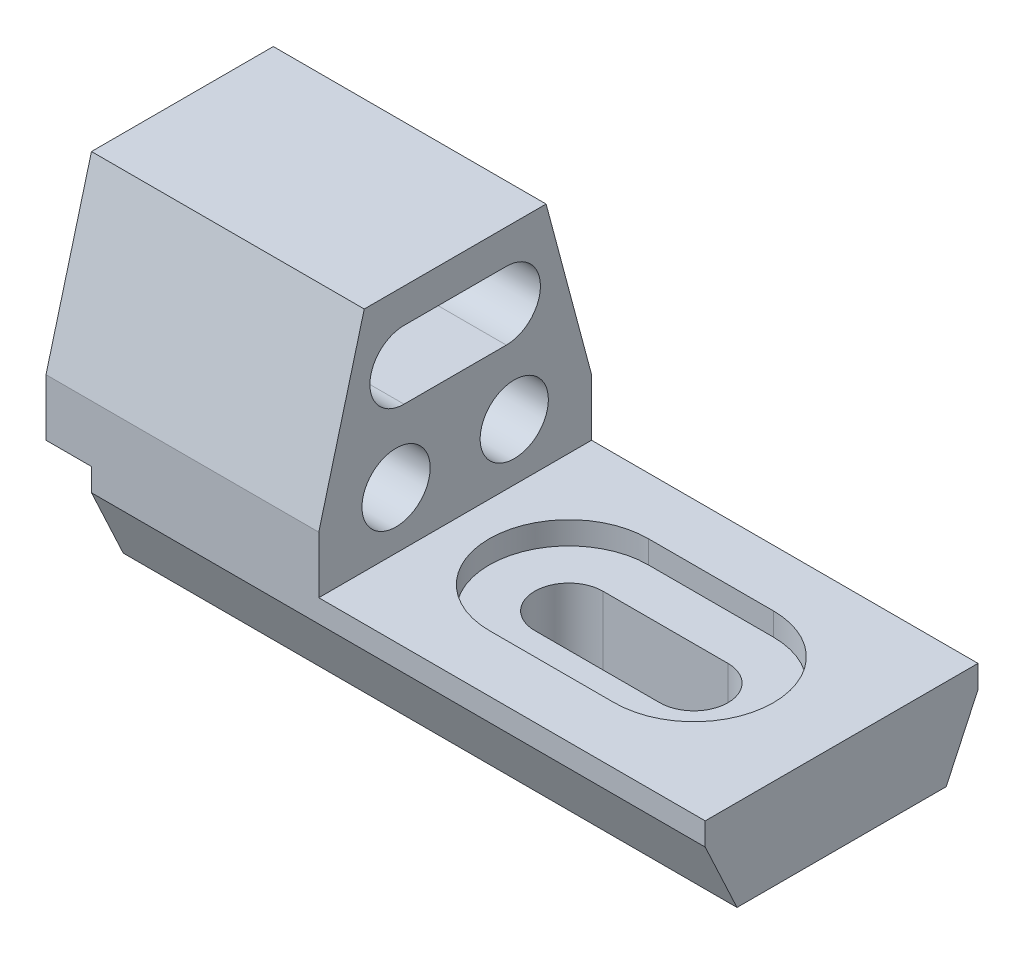
ISO-10303-21;
HEADER;
FILE_DESCRIPTION(('STEP AP214'),'2;1');
FILE_NAME('part.step','',(''),(''),'','','');
FILE_SCHEMA(('AUTOMOTIVE_DESIGN { 1 0 10303 214 1 1 1 1 }'));
ENDSEC;
DATA;
#1=APPLICATION_CONTEXT('core data for automotive mechanical design processes');
#2=APPLICATION_PROTOCOL_DEFINITION('international standard','automotive_design',2000,#1);
#3=PRODUCT_CONTEXT('',#1,'mechanical');
#4=PRODUCT('Part','Part','',(#3));
#5=PRODUCT_RELATED_PRODUCT_CATEGORY('part','',(#4));
#6=PRODUCT_DEFINITION_FORMATION('','',#4);
#7=PRODUCT_DEFINITION_CONTEXT('part definition',#1,'design');
#8=PRODUCT_DEFINITION('design','',#6,#7);
#9=PRODUCT_DEFINITION_SHAPE('','',#8);
#10=(LENGTH_UNIT() NAMED_UNIT(*) SI_UNIT(.MILLI.,.METRE.));
#11=(NAMED_UNIT(*) PLANE_ANGLE_UNIT() SI_UNIT($,.RADIAN.));
#12=(NAMED_UNIT(*) SI_UNIT($,.STERADIAN.) SOLID_ANGLE_UNIT());
#13=UNCERTAINTY_MEASURE_WITH_UNIT(LENGTH_MEASURE(1.E-05),#10,'distance_accuracy_value','');
#14=(GEOMETRIC_REPRESENTATION_CONTEXT(3) GLOBAL_UNCERTAINTY_ASSIGNED_CONTEXT((#13)) GLOBAL_UNIT_ASSIGNED_CONTEXT((#10,
#11,#12)) REPRESENTATION_CONTEXT('',''));
#15=CARTESIAN_POINT('',(0.,0.,0.));
#16=DIRECTION('',(0.,0.,1.));
#17=DIRECTION('',(1.,0.,0.));
#18=AXIS2_PLACEMENT_3D('',#15,#16,#17);
#19=CARTESIAN_POINT('',(135.,0.,-60.));
#20=DIRECTION('',(0.,0.,1.));
#21=DIRECTION('',(1.,0.,0.));
#22=AXIS2_PLACEMENT_3D('',#19,#20,#21);
#23=PLANE('',#22);
#24=DIRECTION('',(0.,1.,0.));
#25=VECTOR('',#24,1.);
#26=CARTESIAN_POINT('',(-135.,0.,-60.));
#27=LINE('',#26,#25);
#28=CARTESIAN_POINT('',(-135.,-9.99999999999999,-60.));
#29=VERTEX_POINT('',#28);
#30=CARTESIAN_POINT('',(-135.,0.,-60.));
#31=VERTEX_POINT('',#30);
#32=EDGE_CURVE('E353',#29,#31,#27,.T.);
#33=ORIENTED_EDGE('',*,*,#32,.T.);
#34=DIRECTION('',(-1.,0.,0.));
#35=VECTOR('',#34,1.);
#36=CARTESIAN_POINT('',(-35.,0.,-60.));
#37=LINE('',#36,#35);
#38=CARTESIAN_POINT('',(-155.,0.,-60.));
#39=VERTEX_POINT('',#38);
#40=EDGE_CURVE('E349',#31,#39,#37,.T.);
#41=ORIENTED_EDGE('',*,*,#40,.T.);
#42=DIRECTION('',(0.,-1.,0.));
#43=VECTOR('',#42,1.);
#44=CARTESIAN_POINT('',(-155.,0.,-60.));
#45=LINE('',#44,#43);
#46=CARTESIAN_POINT('',(-155.,25.,-60.));
#47=VERTEX_POINT('',#46);
#48=EDGE_CURVE('E320',#47,#39,#45,.T.);
#49=ORIENTED_EDGE('',*,*,#48,.F.);
#50=DIRECTION('',(-1.,0.,0.));
#51=VECTOR('',#50,1.);
#52=CARTESIAN_POINT('',(-35.,25.,-60.));
#53=LINE('',#52,#51);
#54=CARTESIAN_POINT('',(-35.,25.,-60.));
#55=VERTEX_POINT('',#54);
#56=EDGE_CURVE('E354',#55,#47,#53,.T.);
#57=ORIENTED_EDGE('',*,*,#56,.F.);
#58=DIRECTION('',(0.,-1.,0.));
#59=VECTOR('',#58,1.);
#60=CARTESIAN_POINT('',(-35.,0.,-60.));
#61=LINE('',#60,#59);
#62=CARTESIAN_POINT('',(-35.,0.,-60.));
#63=VERTEX_POINT('',#62);
#64=EDGE_CURVE('E328',#55,#63,#61,.T.);
#65=ORIENTED_EDGE('',*,*,#64,.T.);
#66=DIRECTION('',(-1.,0.,0.));
#67=VECTOR('',#66,1.);
#68=CARTESIAN_POINT('',(135.,0.,-60.));
#69=LINE('',#68,#67);
#70=CARTESIAN_POINT('',(135.,0.,-60.));
#71=VERTEX_POINT('',#70);
#72=EDGE_CURVE('E11',#71,#63,#69,.T.);
#73=ORIENTED_EDGE('',*,*,#72,.F.);
#74=DIRECTION('',(0.,1.,0.));
#75=VECTOR('',#74,1.);
#76=CARTESIAN_POINT('',(135.,0.,-60.));
#77=LINE('',#76,#75);
#78=CARTESIAN_POINT('',(135.,-9.99999999999999,-60.));
#79=VERTEX_POINT('',#78);
#80=EDGE_CURVE('E363',#79,#71,#77,.T.);
#81=ORIENTED_EDGE('',*,*,#80,.F.);
#82=DIRECTION('',(-1.,0.,0.));
#83=VECTOR('',#82,1.);
#84=CARTESIAN_POINT('',(135.,-9.99999999999999,-60.));
#85=LINE('',#84,#83);
#86=EDGE_CURVE('E374',#79,#29,#85,.T.);
#87=ORIENTED_EDGE('',*,*,#86,.T.);
#88=EDGE_LOOP('',(#33,#41,#49,#57,#65,#73,#81,#87));
#89=FACE_BOUND('',#88,.T.);
#90=ADVANCED_FACE('F39',(#89),#23,.F.);
#91=CARTESIAN_POINT('',(135.,0.,60.));
#92=DIRECTION('',(0.,-1.,0.));
#93=DIRECTION('',(0.,0.,-1.));
#94=AXIS2_PLACEMENT_3D('',#91,#92,#93);
#95=PLANE('',#94);
#96=DIRECTION('',(1.,0.,0.));
#97=VECTOR('',#96,1.);
#98=CARTESIAN_POINT('',(15.,0.,35.));
#99=LINE('',#98,#97);
#100=CARTESIAN_POINT('',(15.,0.,35.));
#101=VERTEX_POINT('',#100);
#102=CARTESIAN_POINT('',(70.,0.,35.));
#103=VERTEX_POINT('',#102);
#104=EDGE_CURVE('E252',#101,#103,#99,.T.);
#105=ORIENTED_EDGE('',*,*,#104,.F.);
#106=CARTESIAN_POINT('',(15.,0.,0.));
#107=DIRECTION('',(0.,1.,0.));
#108=DIRECTION('',(0.,0.,1.));
#109=AXIS2_PLACEMENT_3D('',#106,#107,#108);
#110=CIRCLE('',#109,35.);
#111=CARTESIAN_POINT('',(15.,0.,-35.));
#112=VERTEX_POINT('',#111);
#113=EDGE_CURVE('E235',#112,#101,#110,.T.);
#114=ORIENTED_EDGE('',*,*,#113,.F.);
#115=DIRECTION('',(-1.,0.,0.));
#116=VECTOR('',#115,1.);
#117=CARTESIAN_POINT('',(15.,0.,-35.));
#118=LINE('',#117,#116);
#119=CARTESIAN_POINT('',(70.,0.,-35.));
#120=VERTEX_POINT('',#119);
#121=EDGE_CURVE('E243',#120,#112,#118,.T.);
#122=ORIENTED_EDGE('',*,*,#121,.F.);
#123=CARTESIAN_POINT('',(70.,0.,0.));
#124=DIRECTION('',(0.,1.,0.));
#125=DIRECTION('',(0.,0.,1.));
#126=AXIS2_PLACEMENT_3D('',#123,#124,#125);
#127=CIRCLE('',#126,35.);
#128=EDGE_CURVE('E254',#103,#120,#127,.T.);
#129=ORIENTED_EDGE('',*,*,#128,.F.);
#130=EDGE_LOOP('',(#105,#114,#122,#129));
#131=FACE_BOUND('',#130,.T.);
#132=ORIENTED_EDGE('',*,*,#72,.T.);
#133=DIRECTION('',(0.,0.,1.));
#134=VECTOR('',#133,1.);
#135=CARTESIAN_POINT('',(-35.,0.,-60.));
#136=LINE('',#135,#134);
#137=CARTESIAN_POINT('',(-35.,0.,60.));
#138=VERTEX_POINT('',#137);
#139=EDGE_CURVE('E311',#63,#138,#136,.T.);
#140=ORIENTED_EDGE('',*,*,#139,.T.);
#141=DIRECTION('',(-1.,0.,0.));
#142=VECTOR('',#141,1.);
#143=CARTESIAN_POINT('',(135.,0.,60.));
#144=LINE('',#143,#142);
#145=CARTESIAN_POINT('',(135.,0.,60.));
#146=VERTEX_POINT('',#145);
#147=EDGE_CURVE('E46',#146,#138,#144,.T.);
#148=ORIENTED_EDGE('',*,*,#147,.F.);
#149=DIRECTION('',(0.,0.,1.));
#150=VECTOR('',#149,1.);
#151=CARTESIAN_POINT('',(135.,0.,60.));
#152=LINE('',#151,#150);
#153=EDGE_CURVE('E365',#71,#146,#152,.T.);
#154=ORIENTED_EDGE('',*,*,#153,.F.);
#155=EDGE_LOOP('',(#132,#140,#148,#154));
#156=FACE_BOUND('',#155,.T.);
#157=ADVANCED_FACE('F404',(#131,#156),#95,.F.);
#158=CARTESIAN_POINT('',(135.,0.,60.));
#159=DIRECTION('',(0.,0.,-1.));
#160=DIRECTION('',(-1.,0.,0.));
#161=AXIS2_PLACEMENT_3D('',#158,#159,#160);
#162=PLANE('',#161);
#163=DIRECTION('',(0.,-1.,0.));
#164=VECTOR('',#163,1.);
#165=CARTESIAN_POINT('',(-135.,0.,60.));
#166=LINE('',#165,#164);
#167=CARTESIAN_POINT('',(-135.,0.,60.));
#168=VERTEX_POINT('',#167);
#169=CARTESIAN_POINT('',(-135.,-10.,60.));
#170=VERTEX_POINT('',#169);
#171=EDGE_CURVE('E379',#168,#170,#166,.T.);
#172=ORIENTED_EDGE('',*,*,#171,.T.);
#173=DIRECTION('',(-1.,0.,0.));
#174=VECTOR('',#173,1.);
#175=CARTESIAN_POINT('',(135.,-10.,60.));
#176=LINE('',#175,#174);
#177=CARTESIAN_POINT('',(135.,-10.,60.));
#178=VERTEX_POINT('',#177);
#179=EDGE_CURVE('E391',#178,#170,#176,.T.);
#180=ORIENTED_EDGE('',*,*,#179,.F.);
#181=DIRECTION('',(0.,-1.,0.));
#182=VECTOR('',#181,1.);
#183=CARTESIAN_POINT('',(135.,0.,60.));
#184=LINE('',#183,#182);
#185=EDGE_CURVE('E370',#146,#178,#184,.T.);
#186=ORIENTED_EDGE('',*,*,#185,.F.);
#187=ORIENTED_EDGE('',*,*,#147,.T.);
#188=DIRECTION('',(0.,1.,0.));
#189=VECTOR('',#188,1.);
#190=CARTESIAN_POINT('',(-35.,25.,60.));
#191=LINE('',#190,#189);
#192=CARTESIAN_POINT('',(-35.,25.,60.));
#193=VERTEX_POINT('',#192);
#194=EDGE_CURVE('E316',#138,#193,#191,.T.);
#195=ORIENTED_EDGE('',*,*,#194,.T.);
#196=DIRECTION('',(-1.,0.,0.));
#197=VECTOR('',#196,1.);
#198=CARTESIAN_POINT('',(-35.,25.,60.));
#199=LINE('',#198,#197);
#200=CARTESIAN_POINT('',(-155.,25.,60.));
#201=VERTEX_POINT('',#200);
#202=EDGE_CURVE('E360',#193,#201,#199,.T.);
#203=ORIENTED_EDGE('',*,*,#202,.T.);
#204=DIRECTION('',(0.,1.,0.));
#205=VECTOR('',#204,1.);
#206=CARTESIAN_POINT('',(-155.,25.,60.));
#207=LINE('',#206,#205);
#208=CARTESIAN_POINT('',(-155.,0.,60.));
#209=VERTEX_POINT('',#208);
#210=EDGE_CURVE('E333',#209,#201,#207,.T.);
#211=ORIENTED_EDGE('',*,*,#210,.F.);
#212=DIRECTION('',(-1.,0.,0.));
#213=VECTOR('',#212,1.);
#214=CARTESIAN_POINT('',(-35.,0.,60.));
#215=LINE('',#214,#213);
#216=EDGE_CURVE('E335',#168,#209,#215,.T.);
#217=ORIENTED_EDGE('',*,*,#216,.F.);
#218=EDGE_LOOP('',(#172,#180,#186,#187,#195,#203,#211,#217));
#219=FACE_BOUND('',#218,.T.);
#220=ADVANCED_FACE('F402',(#219),#162,.F.);
#221=CARTESIAN_POINT('',(135.,-10.,60.));
#222=DIRECTION('',(0.,0.422618261740698,-0.906307787036651));
#223=DIRECTION('',(0.,0.906307787036651,0.422618261740698));
#224=AXIS2_PLACEMENT_3D('',#221,#222,#223);
#225=PLANE('',#224);
#226=DIRECTION('',(0.,-0.906307787036651,-0.422618261740698));
#227=VECTOR('',#226,1.);
#228=CARTESIAN_POINT('',(-135.,-10.,60.));
#229=LINE('',#228,#227);
#230=CARTESIAN_POINT('',(-135.,-40.,46.0107702553501));
#231=VERTEX_POINT('',#230);
#232=EDGE_CURVE('E385',#170,#231,#229,.T.);
#233=ORIENTED_EDGE('',*,*,#232,.T.);
#234=DIRECTION('',(-1.,0.,0.));
#235=VECTOR('',#234,1.);
#236=CARTESIAN_POINT('',(135.,-40.,46.0107702553501));
#237=LINE('',#236,#235);
#238=CARTESIAN_POINT('',(135.,-40.,46.0107702553501));
#239=VERTEX_POINT('',#238);
#240=EDGE_CURVE('E394',#239,#231,#237,.T.);
#241=ORIENTED_EDGE('',*,*,#240,.F.);
#242=DIRECTION('',(0.,-0.906307787036651,-0.422618261740698));
#243=VECTOR('',#242,1.);
#244=CARTESIAN_POINT('',(135.,-10.,60.));
#245=LINE('',#244,#243);
#246=EDGE_CURVE('E369',#178,#239,#245,.T.);
#247=ORIENTED_EDGE('',*,*,#246,.F.);
#248=ORIENTED_EDGE('',*,*,#179,.T.);
#249=EDGE_LOOP('',(#233,#241,#247,#248));
#250=FACE_BOUND('',#249,.T.);
#251=ADVANCED_FACE('F447',(#250),#225,.F.);
#252=CARTESIAN_POINT('',(135.,-40.,-46.0107702553501));
#253=DIRECTION('',(0.,1.,0.));
#254=DIRECTION('',(0.,0.,1.));
#255=AXIS2_PLACEMENT_3D('',#252,#253,#254);
#256=PLANE('',#255);
#257=DIRECTION('',(-1.,0.,0.));
#258=VECTOR('',#257,1.);
#259=CARTESIAN_POINT('',(15.,-40.,-15.));
#260=LINE('',#259,#258);
#261=CARTESIAN_POINT('',(70.,-40.,-15.));
#262=VERTEX_POINT('',#261);
#263=CARTESIAN_POINT('',(15.,-40.,-15.));
#264=VERTEX_POINT('',#263);
#265=EDGE_CURVE('E209',#262,#264,#260,.T.);
#266=ORIENTED_EDGE('',*,*,#265,.T.);
#267=CARTESIAN_POINT('',(15.,-40.,0.));
#268=DIRECTION('',(0.,1.,0.));
#269=DIRECTION('',(0.,0.,1.));
#270=AXIS2_PLACEMENT_3D('',#267,#268,#269);
#271=CIRCLE('',#270,15.);
#272=CARTESIAN_POINT('',(15.,-40.,15.));
#273=VERTEX_POINT('',#272);
#274=EDGE_CURVE('E205',#264,#273,#271,.T.);
#275=ORIENTED_EDGE('',*,*,#274,.T.);
#276=DIRECTION('',(1.,0.,0.));
#277=VECTOR('',#276,1.);
#278=CARTESIAN_POINT('',(15.,-40.,15.));
#279=LINE('',#278,#277);
#280=CARTESIAN_POINT('',(70.,-40.,15.));
#281=VERTEX_POINT('',#280);
#282=EDGE_CURVE('E213',#273,#281,#279,.T.);
#283=ORIENTED_EDGE('',*,*,#282,.T.);
#284=CARTESIAN_POINT('',(70.,-40.,0.));
#285=DIRECTION('',(0.,1.,0.));
#286=DIRECTION('',(0.,0.,1.));
#287=AXIS2_PLACEMENT_3D('',#284,#285,#286);
#288=CIRCLE('',#287,15.);
#289=EDGE_CURVE('E59',#281,#262,#288,.T.);
#290=ORIENTED_EDGE('',*,*,#289,.T.);
#291=EDGE_LOOP('',(#266,#275,#283,#290));
#292=FACE_BOUND('',#291,.T.);
#293=DIRECTION('',(0.,0.,-1.));
#294=VECTOR('',#293,1.);
#295=CARTESIAN_POINT('',(-135.,-40.,-46.0107702553501));
#296=LINE('',#295,#294);
#297=CARTESIAN_POINT('',(-135.,-40.,-46.0107702553501));
#298=VERTEX_POINT('',#297);
#299=EDGE_CURVE('E383',#231,#298,#296,.T.);
#300=ORIENTED_EDGE('',*,*,#299,.T.);
#301=DIRECTION('',(-1.,0.,0.));
#302=VECTOR('',#301,1.);
#303=CARTESIAN_POINT('',(135.,-40.,-46.0107702553501));
#304=LINE('',#303,#302);
#305=CARTESIAN_POINT('',(135.,-40.,-46.0107702553501));
#306=VERTEX_POINT('',#305);
#307=EDGE_CURVE('E386',#306,#298,#304,.T.);
#308=ORIENTED_EDGE('',*,*,#307,.F.);
#309=DIRECTION('',(0.,0.,-1.));
#310=VECTOR('',#309,1.);
#311=CARTESIAN_POINT('',(135.,-40.,-46.0107702553501));
#312=LINE('',#311,#310);
#313=EDGE_CURVE('E371',#239,#306,#312,.T.);
#314=ORIENTED_EDGE('',*,*,#313,.F.);
#315=ORIENTED_EDGE('',*,*,#240,.T.);
#316=EDGE_LOOP('',(#300,#308,#314,#315));
#317=FACE_BOUND('',#316,.T.);
#318=ADVANCED_FACE('F220',(#292,#317),#256,.F.);
#319=CARTESIAN_POINT('',(135.,-9.99999999999999,-60.));
#320=DIRECTION('',(0.,0.422618261740697,0.906307787036651));
#321=DIRECTION('',(0.,-0.906307787036651,0.422618261740697));
#322=AXIS2_PLACEMENT_3D('',#319,#320,#321);
#323=PLANE('',#322);
#324=DIRECTION('',(0.,0.906307787036651,-0.422618261740697));
#325=VECTOR('',#324,1.);
#326=CARTESIAN_POINT('',(-135.,-9.99999999999999,-60.));
#327=LINE('',#326,#325);
#328=EDGE_CURVE('E364',#298,#29,#327,.T.);
#329=ORIENTED_EDGE('',*,*,#328,.T.);
#330=ORIENTED_EDGE('',*,*,#86,.F.);
#331=DIRECTION('',(0.,0.906307787036651,-0.422618261740697));
#332=VECTOR('',#331,1.);
#333=CARTESIAN_POINT('',(135.,-9.99999999999999,-60.));
#334=LINE('',#333,#332);
#335=EDGE_CURVE('E373',#306,#79,#334,.T.);
#336=ORIENTED_EDGE('',*,*,#335,.F.);
#337=ORIENTED_EDGE('',*,*,#307,.T.);
#338=EDGE_LOOP('',(#329,#330,#336,#337));
#339=FACE_BOUND('',#338,.T.);
#340=ADVANCED_FACE('F442',(#339),#323,.F.);
#341=CARTESIAN_POINT('',(135.,0.,0.));
#342=DIRECTION('',(-1.,0.,0.));
#343=DIRECTION('',(0.,0.,1.));
#344=AXIS2_PLACEMENT_3D('',#341,#342,#343);
#345=PLANE('',#344);
#346=ORIENTED_EDGE('',*,*,#80,.T.);
#347=ORIENTED_EDGE('',*,*,#153,.T.);
#348=ORIENTED_EDGE('',*,*,#185,.T.);
#349=ORIENTED_EDGE('',*,*,#246,.T.);
#350=ORIENTED_EDGE('',*,*,#313,.T.);
#351=ORIENTED_EDGE('',*,*,#335,.T.);
#352=EDGE_LOOP('',(#346,#347,#348,#349,#350,#351));
#353=FACE_BOUND('',#352,.T.);
#354=ADVANCED_FACE('F446',(#353),#345,.F.);
#355=CARTESIAN_POINT('',(-135.,0.,0.));
#356=DIRECTION('',(-1.,0.,0.));
#357=DIRECTION('',(0.,0.,1.));
#358=AXIS2_PLACEMENT_3D('',#355,#356,#357);
#359=PLANE('',#358);
#360=ORIENTED_EDGE('',*,*,#32,.F.);
#361=ORIENTED_EDGE('',*,*,#328,.F.);
#362=ORIENTED_EDGE('',*,*,#299,.F.);
#363=ORIENTED_EDGE('',*,*,#232,.F.);
#364=ORIENTED_EDGE('',*,*,#171,.F.);
#365=DIRECTION('',(0.,0.,1.));
#366=VECTOR('',#365,1.);
#367=CARTESIAN_POINT('',(-135.,0.,60.));
#368=LINE('',#367,#366);
#369=EDGE_CURVE('E378',#31,#168,#368,.T.);
#370=ORIENTED_EDGE('',*,*,#369,.F.);
#371=EDGE_LOOP('',(#360,#361,#362,#363,#364,#370));
#372=FACE_BOUND('',#371,.T.);
#373=ADVANCED_FACE('F434',(#372),#359,.T.);
#374=CARTESIAN_POINT('',(-35.,0.,-60.));
#375=DIRECTION('',(0.,-1.,0.));
#376=DIRECTION('',(0.,0.,-1.));
#377=AXIS2_PLACEMENT_3D('',#374,#375,#376);
#378=PLANE('',#377);
#379=ORIENTED_EDGE('',*,*,#40,.F.);
#380=ORIENTED_EDGE('',*,*,#369,.T.);
#381=ORIENTED_EDGE('',*,*,#216,.T.);
#382=DIRECTION('',(0.,0.,1.));
#383=VECTOR('',#382,1.);
#384=CARTESIAN_POINT('',(-155.,0.,-60.));
#385=LINE('',#384,#383);
#386=EDGE_CURVE('E309',#39,#209,#385,.T.);
#387=ORIENTED_EDGE('',*,*,#386,.F.);
#388=EDGE_LOOP('',(#379,#380,#381,#387));
#389=FACE_BOUND('',#388,.T.);
#390=ADVANCED_FACE('F431',(#389),#378,.T.);
#391=CARTESIAN_POINT('',(-35.,25.,-60.));
#392=DIRECTION('',(0.,0.257662650560332,-0.966234939601246));
#393=DIRECTION('',(0.,0.966234939601246,0.257662650560332));
#394=AXIS2_PLACEMENT_3D('',#391,#392,#393);
#395=PLANE('',#394);
#396=DIRECTION('',(0.,-0.966234939601246,-0.257662650560332));
#397=VECTOR('',#396,1.);
#398=CARTESIAN_POINT('',(-155.,25.,-60.));
#399=LINE('',#398,#397);
#400=CARTESIAN_POINT('',(-155.,100.,-40.));
#401=VERTEX_POINT('',#400);
#402=EDGE_CURVE('E341',#401,#47,#399,.T.);
#403=ORIENTED_EDGE('',*,*,#402,.F.);
#404=DIRECTION('',(-1.,0.,0.));
#405=VECTOR('',#404,1.);
#406=CARTESIAN_POINT('',(-35.,100.,-40.));
#407=LINE('',#406,#405);
#408=CARTESIAN_POINT('',(-35.,100.,-40.));
#409=VERTEX_POINT('',#408);
#410=EDGE_CURVE('E355',#409,#401,#407,.T.);
#411=ORIENTED_EDGE('',*,*,#410,.F.);
#412=DIRECTION('',(0.,-0.966234939601246,-0.257662650560332));
#413=VECTOR('',#412,1.);
#414=CARTESIAN_POINT('',(-35.,25.,-60.));
#415=LINE('',#414,#413);
#416=EDGE_CURVE('E326',#409,#55,#415,.T.);
#417=ORIENTED_EDGE('',*,*,#416,.T.);
#418=ORIENTED_EDGE('',*,*,#56,.T.);
#419=EDGE_LOOP('',(#403,#411,#417,#418));
#420=FACE_BOUND('',#419,.T.);
#421=ADVANCED_FACE('F418',(#420),#395,.T.);
#422=CARTESIAN_POINT('',(-35.,100.,-40.));
#423=DIRECTION('',(0.,1.,0.));
#424=DIRECTION('',(0.,0.,1.));
#425=AXIS2_PLACEMENT_3D('',#422,#423,#424);
#426=PLANE('',#425);
#427=DIRECTION('',(0.,0.,-1.));
#428=VECTOR('',#427,1.);
#429=CARTESIAN_POINT('',(-155.,100.,-40.));
#430=LINE('',#429,#428);
#431=CARTESIAN_POINT('',(-155.,100.,40.));
#432=VERTEX_POINT('',#431);
#433=EDGE_CURVE('E342',#432,#401,#430,.T.);
#434=ORIENTED_EDGE('',*,*,#433,.F.);
#435=DIRECTION('',(-1.,0.,0.));
#436=VECTOR('',#435,1.);
#437=CARTESIAN_POINT('',(-35.,100.,40.));
#438=LINE('',#437,#436);
#439=CARTESIAN_POINT('',(-35.,100.,40.));
#440=VERTEX_POINT('',#439);
#441=EDGE_CURVE('E357',#440,#432,#438,.T.);
#442=ORIENTED_EDGE('',*,*,#441,.F.);
#443=DIRECTION('',(0.,0.,-1.));
#444=VECTOR('',#443,1.);
#445=CARTESIAN_POINT('',(-35.,100.,-40.));
#446=LINE('',#445,#444);
#447=EDGE_CURVE('E323',#440,#409,#446,.T.);
#448=ORIENTED_EDGE('',*,*,#447,.T.);
#449=ORIENTED_EDGE('',*,*,#410,.T.);
#450=EDGE_LOOP('',(#434,#442,#448,#449));
#451=FACE_BOUND('',#450,.T.);
#452=ADVANCED_FACE('F419',(#451),#426,.T.);
#453=CARTESIAN_POINT('',(-35.,100.,40.));
#454=DIRECTION('',(0.,0.257662650560332,0.966234939601246));
#455=DIRECTION('',(0.,-0.966234939601246,0.257662650560332));
#456=AXIS2_PLACEMENT_3D('',#453,#454,#455);
#457=PLANE('',#456);
#458=DIRECTION('',(0.,0.966234939601246,-0.257662650560332));
#459=VECTOR('',#458,1.);
#460=CARTESIAN_POINT('',(-155.,100.,40.));
#461=LINE('',#460,#459);
#462=EDGE_CURVE('E337',#201,#432,#461,.T.);
#463=ORIENTED_EDGE('',*,*,#462,.F.);
#464=ORIENTED_EDGE('',*,*,#202,.F.);
#465=DIRECTION('',(0.,0.966234939601246,-0.257662650560332));
#466=VECTOR('',#465,1.);
#467=CARTESIAN_POINT('',(-35.,100.,40.));
#468=LINE('',#467,#466);
#469=EDGE_CURVE('E319',#193,#440,#468,.T.);
#470=ORIENTED_EDGE('',*,*,#469,.T.);
#471=ORIENTED_EDGE('',*,*,#441,.T.);
#472=EDGE_LOOP('',(#463,#464,#470,#471));
#473=FACE_BOUND('',#472,.T.);
#474=ADVANCED_FACE('F421',(#473),#457,.T.);
#475=CARTESIAN_POINT('',(-35.,0.,0.));
#476=DIRECTION('',(1.,0.,0.));
#477=DIRECTION('',(0.,0.,-1.));
#478=AXIS2_PLACEMENT_3D('',#475,#476,#477);
#479=PLANE('',#478);
#480=CARTESIAN_POINT('',(-35.,70.,22.5));
#481=DIRECTION('',(1.,0.,0.));
#482=DIRECTION('',(0.,0.,-1.));
#483=AXIS2_PLACEMENT_3D('',#480,#481,#482);
#484=CIRCLE('',#483,15.);
#485=CARTESIAN_POINT('',(-35.,85.,22.5));
#486=VERTEX_POINT('',#485);
#487=CARTESIAN_POINT('',(-35.,55.,22.5));
#488=VERTEX_POINT('',#487);
#489=EDGE_CURVE('E265',#486,#488,#484,.T.);
#490=ORIENTED_EDGE('',*,*,#489,.F.);
#491=DIRECTION('',(0.,0.,1.));
#492=VECTOR('',#491,1.);
#493=CARTESIAN_POINT('',(-35.,85.,22.5));
#494=LINE('',#493,#492);
#495=CARTESIAN_POINT('',(-35.,85.,-22.5));
#496=VERTEX_POINT('',#495);
#497=EDGE_CURVE('E283',#496,#486,#494,.T.);
#498=ORIENTED_EDGE('',*,*,#497,.F.);
#499=CARTESIAN_POINT('',(-35.,70.,-22.5));
#500=DIRECTION('',(1.,0.,0.));
#501=DIRECTION('',(0.,0.,-1.));
#502=AXIS2_PLACEMENT_3D('',#499,#500,#501);
#503=CIRCLE('',#502,15.);
#504=CARTESIAN_POINT('',(-35.,55.,-22.5));
#505=VERTEX_POINT('',#504);
#506=EDGE_CURVE('E293',#505,#496,#503,.T.);
#507=ORIENTED_EDGE('',*,*,#506,.F.);
#508=DIRECTION('',(0.,0.,-1.));
#509=VECTOR('',#508,1.);
#510=CARTESIAN_POINT('',(-35.,55.,22.5));
#511=LINE('',#510,#509);
#512=EDGE_CURVE('E295',#488,#505,#511,.T.);
#513=ORIENTED_EDGE('',*,*,#512,.F.);
#514=EDGE_LOOP('',(#490,#498,#507,#513));
#515=FACE_BOUND('',#514,.T.);
#516=CARTESIAN_POINT('',(-35.,25.,-26.));
#517=DIRECTION('',(1.,0.,0.));
#518=DIRECTION('',(0.,0.,-1.));
#519=AXIS2_PLACEMENT_3D('',#516,#517,#518);
#520=CIRCLE('',#519,15.);
#521=CARTESIAN_POINT('',(-35.,25.,-41.));
#522=VERTEX_POINT('',#521);
#523=EDGE_CURVE('E272',#522,#522,#520,.T.);
#524=ORIENTED_EDGE('',*,*,#523,.F.);
#525=EDGE_LOOP('',(#524));
#526=FACE_BOUND('',#525,.T.);
#527=CARTESIAN_POINT('',(-35.,25.,26.));
#528=DIRECTION('',(1.,0.,0.));
#529=DIRECTION('',(0.,0.,-1.));
#530=AXIS2_PLACEMENT_3D('',#527,#528,#529);
#531=CIRCLE('',#530,15.);
#532=CARTESIAN_POINT('',(-35.,25.,11.));
#533=VERTEX_POINT('',#532);
#534=EDGE_CURVE('E275',#533,#533,#531,.T.);
#535=ORIENTED_EDGE('',*,*,#534,.F.);
#536=EDGE_LOOP('',(#535));
#537=FACE_BOUND('',#536,.T.);
#538=ORIENTED_EDGE('',*,*,#139,.F.);
#539=ORIENTED_EDGE('',*,*,#64,.F.);
#540=ORIENTED_EDGE('',*,*,#416,.F.);
#541=ORIENTED_EDGE('',*,*,#447,.F.);
#542=ORIENTED_EDGE('',*,*,#469,.F.);
#543=ORIENTED_EDGE('',*,*,#194,.F.);
#544=EDGE_LOOP('',(#538,#539,#540,#541,#542,#543));
#545=FACE_BOUND('',#544,.T.);
#546=ADVANCED_FACE('F407',(#515,#526,#537,#545),#479,.T.);
#547=CARTESIAN_POINT('',(-155.,0.,0.));
#548=DIRECTION('',(1.,0.,0.));
#549=DIRECTION('',(0.,0.,-1.));
#550=AXIS2_PLACEMENT_3D('',#547,#548,#549);
#551=PLANE('',#550);
#552=DIRECTION('',(0.,0.,1.));
#553=VECTOR('',#552,1.);
#554=CARTESIAN_POINT('',(-155.,85.,22.5));
#555=LINE('',#554,#553);
#556=CARTESIAN_POINT('',(-155.,85.,-22.5));
#557=VERTEX_POINT('',#556);
#558=CARTESIAN_POINT('',(-155.,85.,22.5));
#559=VERTEX_POINT('',#558);
#560=EDGE_CURVE('E289',#557,#559,#555,.T.);
#561=ORIENTED_EDGE('',*,*,#560,.T.);
#562=CARTESIAN_POINT('',(-155.,70.,22.5));
#563=DIRECTION('',(1.,0.,0.));
#564=DIRECTION('',(0.,0.,-1.));
#565=AXIS2_PLACEMENT_3D('',#562,#563,#564);
#566=CIRCLE('',#565,15.);
#567=CARTESIAN_POINT('',(-155.,55.,22.5));
#568=VERTEX_POINT('',#567);
#569=EDGE_CURVE('E280',#559,#568,#566,.T.);
#570=ORIENTED_EDGE('',*,*,#569,.T.);
#571=DIRECTION('',(0.,0.,-1.));
#572=VECTOR('',#571,1.);
#573=CARTESIAN_POINT('',(-155.,55.,22.5));
#574=LINE('',#573,#572);
#575=CARTESIAN_POINT('',(-155.,55.,-22.5));
#576=VERTEX_POINT('',#575);
#577=EDGE_CURVE('E278',#568,#576,#574,.T.);
#578=ORIENTED_EDGE('',*,*,#577,.T.);
#579=CARTESIAN_POINT('',(-155.,70.,-22.5));
#580=DIRECTION('',(1.,0.,0.));
#581=DIRECTION('',(0.,0.,-1.));
#582=AXIS2_PLACEMENT_3D('',#579,#580,#581);
#583=CIRCLE('',#582,15.);
#584=EDGE_CURVE('E285',#576,#557,#583,.T.);
#585=ORIENTED_EDGE('',*,*,#584,.T.);
#586=EDGE_LOOP('',(#561,#570,#578,#585));
#587=FACE_BOUND('',#586,.T.);
#588=CARTESIAN_POINT('',(-155.,25.,-26.));
#589=DIRECTION('',(1.,0.,0.));
#590=DIRECTION('',(0.,0.,-1.));
#591=AXIS2_PLACEMENT_3D('',#588,#589,#590);
#592=CIRCLE('',#591,15.);
#593=CARTESIAN_POINT('',(-155.,25.,-41.));
#594=VERTEX_POINT('',#593);
#595=EDGE_CURVE('E267',#594,#594,#592,.T.);
#596=ORIENTED_EDGE('',*,*,#595,.T.);
#597=EDGE_LOOP('',(#596));
#598=FACE_BOUND('',#597,.T.);
#599=CARTESIAN_POINT('',(-155.,25.,26.));
#600=DIRECTION('',(1.,0.,0.));
#601=DIRECTION('',(0.,0.,-1.));
#602=AXIS2_PLACEMENT_3D('',#599,#600,#601);
#603=CIRCLE('',#602,15.);
#604=CARTESIAN_POINT('',(-155.,25.,11.));
#605=VERTEX_POINT('',#604);
#606=EDGE_CURVE('E307',#605,#605,#603,.T.);
#607=ORIENTED_EDGE('',*,*,#606,.T.);
#608=EDGE_LOOP('',(#607));
#609=FACE_BOUND('',#608,.T.);
#610=ORIENTED_EDGE('',*,*,#386,.T.);
#611=ORIENTED_EDGE('',*,*,#210,.T.);
#612=ORIENTED_EDGE('',*,*,#462,.T.);
#613=ORIENTED_EDGE('',*,*,#433,.T.);
#614=ORIENTED_EDGE('',*,*,#402,.T.);
#615=ORIENTED_EDGE('',*,*,#48,.T.);
#616=EDGE_LOOP('',(#610,#611,#612,#613,#614,#615));
#617=FACE_BOUND('',#616,.T.);
#618=ADVANCED_FACE('F427',(#587,#598,#609,#617),#551,.F.);
#619=CARTESIAN_POINT('',(-155.,25.,26.));
#620=DIRECTION('',(1.,0.,0.));
#621=DIRECTION('',(0.,0.,-1.));
#622=AXIS2_PLACEMENT_3D('',#619,#620,#621);
#623=CYLINDRICAL_SURFACE('',#622,15.);
#624=ORIENTED_EDGE('',*,*,#606,.F.);
#625=EDGE_LOOP('',(#624));
#626=FACE_BOUND('',#625,.T.);
#627=ORIENTED_EDGE('',*,*,#534,.T.);
#628=EDGE_LOOP('',(#627));
#629=FACE_BOUND('',#628,.T.);
#630=ADVANCED_FACE('F604',(#626,#629),#623,.F.);
#631=CARTESIAN_POINT('',(-155.,25.,-26.));
#632=DIRECTION('',(1.,0.,0.));
#633=DIRECTION('',(0.,0.,-1.));
#634=AXIS2_PLACEMENT_3D('',#631,#632,#633);
#635=CYLINDRICAL_SURFACE('',#634,15.);
#636=ORIENTED_EDGE('',*,*,#595,.F.);
#637=EDGE_LOOP('',(#636));
#638=FACE_BOUND('',#637,.T.);
#639=ORIENTED_EDGE('',*,*,#523,.T.);
#640=EDGE_LOOP('',(#639));
#641=FACE_BOUND('',#640,.T.);
#642=ADVANCED_FACE('F596',(#638,#641),#635,.F.);
#643=CARTESIAN_POINT('',(-155.,70.,22.5));
#644=DIRECTION('',(1.,0.,0.));
#645=DIRECTION('',(0.,0.,-1.));
#646=AXIS2_PLACEMENT_3D('',#643,#644,#645);
#647=CYLINDRICAL_SURFACE('',#646,15.);
#648=ORIENTED_EDGE('',*,*,#489,.T.);
#649=DIRECTION('',(1.,0.,0.));
#650=VECTOR('',#649,1.);
#651=CARTESIAN_POINT('',(-155.,55.,22.5));
#652=LINE('',#651,#650);
#653=EDGE_CURVE('E288',#568,#488,#652,.T.);
#654=ORIENTED_EDGE('',*,*,#653,.F.);
#655=ORIENTED_EDGE('',*,*,#569,.F.);
#656=DIRECTION('',(1.,0.,0.));
#657=VECTOR('',#656,1.);
#658=CARTESIAN_POINT('',(-155.,85.,22.5));
#659=LINE('',#658,#657);
#660=EDGE_CURVE('E277',#559,#486,#659,.T.);
#661=ORIENTED_EDGE('',*,*,#660,.T.);
#662=EDGE_LOOP('',(#648,#654,#655,#661));
#663=FACE_BOUND('',#662,.T.);
#664=ADVANCED_FACE('F590',(#663),#647,.F.);
#665=CARTESIAN_POINT('',(-155.,85.,22.5));
#666=DIRECTION('',(0.,1.,0.));
#667=DIRECTION('',(0.,0.,1.));
#668=AXIS2_PLACEMENT_3D('',#665,#666,#667);
#669=PLANE('',#668);
#670=ORIENTED_EDGE('',*,*,#497,.T.);
#671=ORIENTED_EDGE('',*,*,#660,.F.);
#672=ORIENTED_EDGE('',*,*,#560,.F.);
#673=DIRECTION('',(1.,0.,0.));
#674=VECTOR('',#673,1.);
#675=CARTESIAN_POINT('',(-155.,85.,-22.5));
#676=LINE('',#675,#674);
#677=EDGE_CURVE('E302',#557,#496,#676,.T.);
#678=ORIENTED_EDGE('',*,*,#677,.T.);
#679=EDGE_LOOP('',(#670,#671,#672,#678));
#680=FACE_BOUND('',#679,.T.);
#681=ADVANCED_FACE('F580',(#680),#669,.F.);
#682=CARTESIAN_POINT('',(-155.,70.,-22.5));
#683=DIRECTION('',(1.,0.,0.));
#684=DIRECTION('',(0.,0.,-1.));
#685=AXIS2_PLACEMENT_3D('',#682,#683,#684);
#686=CYLINDRICAL_SURFACE('',#685,15.);
#687=ORIENTED_EDGE('',*,*,#506,.T.);
#688=ORIENTED_EDGE('',*,*,#677,.F.);
#689=ORIENTED_EDGE('',*,*,#584,.F.);
#690=DIRECTION('',(1.,0.,0.));
#691=VECTOR('',#690,1.);
#692=CARTESIAN_POINT('',(-155.,55.,-22.5));
#693=LINE('',#692,#691);
#694=EDGE_CURVE('E305',#576,#505,#693,.T.);
#695=ORIENTED_EDGE('',*,*,#694,.T.);
#696=EDGE_LOOP('',(#687,#688,#689,#695));
#697=FACE_BOUND('',#696,.T.);
#698=ADVANCED_FACE('F569',(#697),#686,.F.);
#699=CARTESIAN_POINT('',(-155.,55.,22.5));
#700=DIRECTION('',(0.,-1.,0.));
#701=DIRECTION('',(0.,0.,-1.));
#702=AXIS2_PLACEMENT_3D('',#699,#700,#701);
#703=PLANE('',#702);
#704=ORIENTED_EDGE('',*,*,#512,.T.);
#705=ORIENTED_EDGE('',*,*,#694,.F.);
#706=ORIENTED_EDGE('',*,*,#577,.F.);
#707=ORIENTED_EDGE('',*,*,#653,.T.);
#708=EDGE_LOOP('',(#704,#705,#706,#707));
#709=FACE_BOUND('',#708,.T.);
#710=ADVANCED_FACE('F562',(#709),#703,.F.);
#711=CARTESIAN_POINT('',(15.,-10.,0.));
#712=DIRECTION('',(0.,1.,0.));
#713=DIRECTION('',(0.,0.,1.));
#714=AXIS2_PLACEMENT_3D('',#711,#712,#713);
#715=CYLINDRICAL_SURFACE('',#714,35.);
#716=ORIENTED_EDGE('',*,*,#113,.T.);
#717=DIRECTION('',(0.,1.,0.));
#718=VECTOR('',#717,1.);
#719=CARTESIAN_POINT('',(15.,-10.,35.));
#720=LINE('',#719,#718);
#721=CARTESIAN_POINT('',(15.,-10.,35.));
#722=VERTEX_POINT('',#721);
#723=EDGE_CURVE('E248',#722,#101,#720,.T.);
#724=ORIENTED_EDGE('',*,*,#723,.F.);
#725=CARTESIAN_POINT('',(15.,-10.,0.));
#726=DIRECTION('',(0.,1.,0.));
#727=DIRECTION('',(0.,0.,1.));
#728=AXIS2_PLACEMENT_3D('',#725,#726,#727);
#729=CIRCLE('',#728,35.);
#730=CARTESIAN_POINT('',(15.,-10.,-35.));
#731=VERTEX_POINT('',#730);
#732=EDGE_CURVE('E240',#731,#722,#729,.T.);
#733=ORIENTED_EDGE('',*,*,#732,.F.);
#734=DIRECTION('',(0.,1.,0.));
#735=VECTOR('',#734,1.);
#736=CARTESIAN_POINT('',(15.,-10.,-35.));
#737=LINE('',#736,#735);
#738=EDGE_CURVE('E257',#731,#112,#737,.T.);
#739=ORIENTED_EDGE('',*,*,#738,.T.);
#740=EDGE_LOOP('',(#716,#724,#733,#739));
#741=FACE_BOUND('',#740,.T.);
#742=ADVANCED_FACE('F554',(#741),#715,.F.);
#743=CARTESIAN_POINT('',(15.,-10.,-35.));
#744=DIRECTION('',(0.,0.,-1.));
#745=DIRECTION('',(0.,1.,0.));
#746=AXIS2_PLACEMENT_3D('',#743,#744,#745);
#747=PLANE('',#746);
#748=ORIENTED_EDGE('',*,*,#121,.T.);
#749=ORIENTED_EDGE('',*,*,#738,.F.);
#750=DIRECTION('',(-1.,0.,0.));
#751=VECTOR('',#750,1.);
#752=CARTESIAN_POINT('',(15.,-10.,-35.));
#753=LINE('',#752,#751);
#754=CARTESIAN_POINT('',(70.,-10.,-35.));
#755=VERTEX_POINT('',#754);
#756=EDGE_CURVE('E249',#755,#731,#753,.T.);
#757=ORIENTED_EDGE('',*,*,#756,.F.);
#758=DIRECTION('',(0.,1.,0.));
#759=VECTOR('',#758,1.);
#760=CARTESIAN_POINT('',(70.,-10.,-35.));
#761=LINE('',#760,#759);
#762=EDGE_CURVE('E263',#755,#120,#761,.T.);
#763=ORIENTED_EDGE('',*,*,#762,.T.);
#764=EDGE_LOOP('',(#748,#749,#757,#763));
#765=FACE_BOUND('',#764,.T.);
#766=ADVANCED_FACE('F542',(#765),#747,.F.);
#767=CARTESIAN_POINT('',(70.,-10.,0.));
#768=DIRECTION('',(0.,1.,0.));
#769=DIRECTION('',(0.,0.,1.));
#770=AXIS2_PLACEMENT_3D('',#767,#768,#769);
#771=CYLINDRICAL_SURFACE('',#770,35.);
#772=ORIENTED_EDGE('',*,*,#128,.T.);
#773=ORIENTED_EDGE('',*,*,#762,.F.);
#774=CARTESIAN_POINT('',(70.,-10.,0.));
#775=DIRECTION('',(0.,1.,0.));
#776=DIRECTION('',(0.,0.,1.));
#777=AXIS2_PLACEMENT_3D('',#774,#775,#776);
#778=CIRCLE('',#777,35.);
#779=CARTESIAN_POINT('',(70.,-10.,35.));
#780=VERTEX_POINT('',#779);
#781=EDGE_CURVE('E245',#780,#755,#778,.T.);
#782=ORIENTED_EDGE('',*,*,#781,.F.);
#783=DIRECTION('',(0.,1.,0.));
#784=VECTOR('',#783,1.);
#785=CARTESIAN_POINT('',(70.,-10.,35.));
#786=LINE('',#785,#784);
#787=EDGE_CURVE('E264',#780,#103,#786,.T.);
#788=ORIENTED_EDGE('',*,*,#787,.T.);
#789=EDGE_LOOP('',(#772,#773,#782,#788));
#790=FACE_BOUND('',#789,.T.);
#791=ADVANCED_FACE('F536',(#790),#771,.F.);
#792=CARTESIAN_POINT('',(15.,-10.,35.));
#793=DIRECTION('',(0.,0.,1.));
#794=DIRECTION('',(0.,-1.,0.));
#795=AXIS2_PLACEMENT_3D('',#792,#793,#794);
#796=PLANE('',#795);
#797=ORIENTED_EDGE('',*,*,#104,.T.);
#798=ORIENTED_EDGE('',*,*,#787,.F.);
#799=DIRECTION('',(1.,0.,0.));
#800=VECTOR('',#799,1.);
#801=CARTESIAN_POINT('',(15.,-10.,35.));
#802=LINE('',#801,#800);
#803=EDGE_CURVE('E238',#722,#780,#802,.T.);
#804=ORIENTED_EDGE('',*,*,#803,.F.);
#805=ORIENTED_EDGE('',*,*,#723,.T.);
#806=EDGE_LOOP('',(#797,#798,#804,#805));
#807=FACE_BOUND('',#806,.T.);
#808=ADVANCED_FACE('F484',(#807),#796,.F.);
#809=CARTESIAN_POINT('',(15.,-10.,0.));
#810=DIRECTION('',(0.,1.,0.));
#811=DIRECTION('',(0.,0.,1.));
#812=AXIS2_PLACEMENT_3D('',#809,#810,#811);
#813=PLANE('',#812);
#814=CARTESIAN_POINT('',(15.,-10.,0.));
#815=DIRECTION('',(0.,1.,0.));
#816=DIRECTION('',(0.,0.,1.));
#817=AXIS2_PLACEMENT_3D('',#814,#815,#816);
#818=CIRCLE('',#817,15.);
#819=CARTESIAN_POINT('',(15.,-10.,-15.));
#820=VERTEX_POINT('',#819);
#821=CARTESIAN_POINT('',(15.,-10.,15.));
#822=VERTEX_POINT('',#821);
#823=EDGE_CURVE('E202',#820,#822,#818,.T.);
#824=ORIENTED_EDGE('',*,*,#823,.F.);
#825=DIRECTION('',(-1.,0.,0.));
#826=VECTOR('',#825,1.);
#827=CARTESIAN_POINT('',(15.,-10.,-15.));
#828=LINE('',#827,#826);
#829=CARTESIAN_POINT('',(70.,-10.,-15.));
#830=VERTEX_POINT('',#829);
#831=EDGE_CURVE('E219',#830,#820,#828,.T.);
#832=ORIENTED_EDGE('',*,*,#831,.F.);
#833=CARTESIAN_POINT('',(70.,-10.,0.));
#834=DIRECTION('',(0.,1.,0.));
#835=DIRECTION('',(0.,0.,1.));
#836=AXIS2_PLACEMENT_3D('',#833,#834,#835);
#837=CIRCLE('',#836,15.);
#838=CARTESIAN_POINT('',(70.,-10.,15.));
#839=VERTEX_POINT('',#838);
#840=EDGE_CURVE('E52',#839,#830,#837,.T.);
#841=ORIENTED_EDGE('',*,*,#840,.F.);
#842=DIRECTION('',(1.,0.,0.));
#843=VECTOR('',#842,1.);
#844=CARTESIAN_POINT('',(15.,-10.,15.));
#845=LINE('',#844,#843);
#846=EDGE_CURVE('E227',#822,#839,#845,.T.);
#847=ORIENTED_EDGE('',*,*,#846,.F.);
#848=EDGE_LOOP('',(#824,#832,#841,#847));
#849=FACE_BOUND('',#848,.T.);
#850=ORIENTED_EDGE('',*,*,#732,.T.);
#851=ORIENTED_EDGE('',*,*,#803,.T.);
#852=ORIENTED_EDGE('',*,*,#781,.T.);
#853=ORIENTED_EDGE('',*,*,#756,.T.);
#854=EDGE_LOOP('',(#850,#851,#852,#853));
#855=FACE_BOUND('',#854,.T.);
#856=ADVANCED_FACE('F487',(#849,#855),#813,.T.);
#857=CARTESIAN_POINT('',(15.,-40.,0.));
#858=DIRECTION('',(0.,1.,0.));
#859=DIRECTION('',(0.,0.,1.));
#860=AXIS2_PLACEMENT_3D('',#857,#858,#859);
#861=CYLINDRICAL_SURFACE('',#860,15.);
#862=ORIENTED_EDGE('',*,*,#823,.T.);
#863=DIRECTION('',(0.,1.,0.));
#864=VECTOR('',#863,1.);
#865=CARTESIAN_POINT('',(15.,-40.,15.));
#866=LINE('',#865,#864);
#867=EDGE_CURVE('E196',#273,#822,#866,.T.);
#868=ORIENTED_EDGE('',*,*,#867,.F.);
#869=ORIENTED_EDGE('',*,*,#274,.F.);
#870=DIRECTION('',(0.,1.,0.));
#871=VECTOR('',#870,1.);
#872=CARTESIAN_POINT('',(15.,-40.,-15.));
#873=LINE('',#872,#871);
#874=EDGE_CURVE('E232',#264,#820,#873,.T.);
#875=ORIENTED_EDGE('',*,*,#874,.T.);
#876=EDGE_LOOP('',(#862,#868,#869,#875));
#877=FACE_BOUND('',#876,.T.);
#878=ADVANCED_FACE('F199',(#877),#861,.F.);
#879=CARTESIAN_POINT('',(15.,-40.,-15.));
#880=DIRECTION('',(0.,0.,-1.));
#881=DIRECTION('',(0.,1.,0.));
#882=AXIS2_PLACEMENT_3D('',#879,#880,#881);
#883=PLANE('',#882);
#884=ORIENTED_EDGE('',*,*,#831,.T.);
#885=ORIENTED_EDGE('',*,*,#874,.F.);
#886=ORIENTED_EDGE('',*,*,#265,.F.);
#887=DIRECTION('',(0.,1.,0.));
#888=VECTOR('',#887,1.);
#889=CARTESIAN_POINT('',(70.,-40.,-15.));
#890=LINE('',#889,#888);
#891=EDGE_CURVE('E231',#262,#830,#890,.T.);
#892=ORIENTED_EDGE('',*,*,#891,.T.);
#893=EDGE_LOOP('',(#884,#885,#886,#892));
#894=FACE_BOUND('',#893,.T.);
#895=ADVANCED_FACE('F503',(#894),#883,.F.);
#896=CARTESIAN_POINT('',(70.,-40.,0.));
#897=DIRECTION('',(0.,1.,0.));
#898=DIRECTION('',(0.,0.,1.));
#899=AXIS2_PLACEMENT_3D('',#896,#897,#898);
#900=CYLINDRICAL_SURFACE('',#899,15.);
#901=ORIENTED_EDGE('',*,*,#840,.T.);
#902=ORIENTED_EDGE('',*,*,#891,.F.);
#903=ORIENTED_EDGE('',*,*,#289,.F.);
#904=DIRECTION('',(0.,1.,0.));
#905=VECTOR('',#904,1.);
#906=CARTESIAN_POINT('',(70.,-40.,15.));
#907=LINE('',#906,#905);
#908=EDGE_CURVE('E207',#281,#839,#907,.T.);
#909=ORIENTED_EDGE('',*,*,#908,.T.);
#910=EDGE_LOOP('',(#901,#902,#903,#909));
#911=FACE_BOUND('',#910,.T.);
#912=ADVANCED_FACE('F506',(#911),#900,.F.);
#913=CARTESIAN_POINT('',(15.,-40.,15.));
#914=DIRECTION('',(0.,0.,1.));
#915=DIRECTION('',(0.,-1.,0.));
#916=AXIS2_PLACEMENT_3D('',#913,#914,#915);
#917=PLANE('',#916);
#918=ORIENTED_EDGE('',*,*,#846,.T.);
#919=ORIENTED_EDGE('',*,*,#908,.F.);
#920=ORIENTED_EDGE('',*,*,#282,.F.);
#921=ORIENTED_EDGE('',*,*,#867,.T.);
#922=EDGE_LOOP('',(#918,#919,#920,#921));
#923=FACE_BOUND('',#922,.T.);
#924=ADVANCED_FACE('F212',(#923),#917,.F.);
#925=CLOSED_SHELL('',(#90,#157,#220,#251,#318,#340,#354,#373,#390,#421,#452,#474,#546,#618,#630,
#642,#664,#681,#698,#710,#742,#766,#791,#808,#856,#878,#895,#912,#924));
#926=MANIFOLD_SOLID_BREP('B2',#925);
#927=ADVANCED_BREP_SHAPE_REPRESENTATION('',(#18,#926),#14);
#928=SHAPE_DEFINITION_REPRESENTATION(#9,#927);
ENDSEC;
END-ISO-10303-21;
